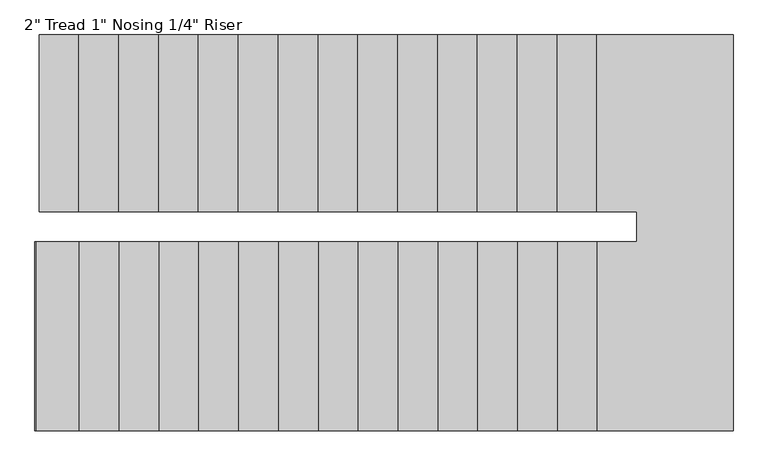
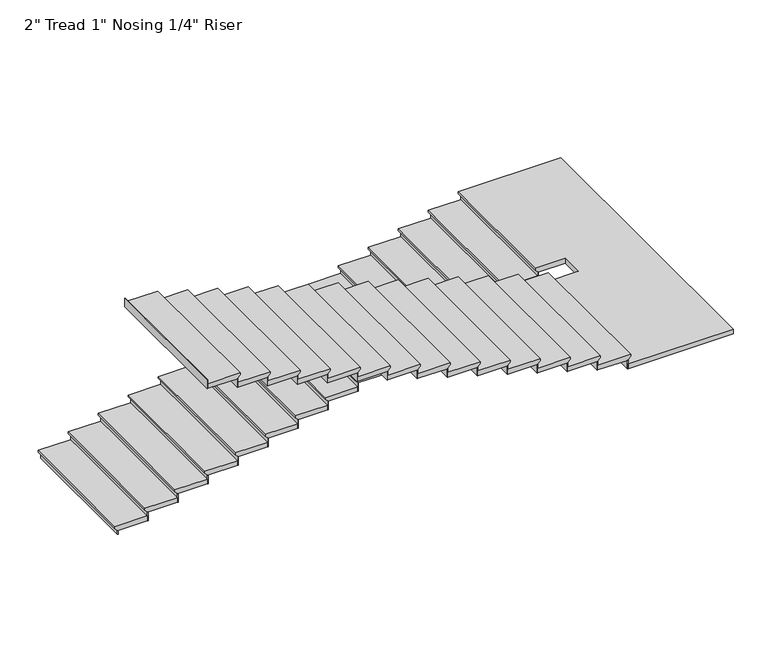
"""IFC4 building model written with IfcOpenShell, lengths in millimetres: stair flight geometry."""

from ifc_helpers import new_model, si_unit, origin, place, context, project, spatial, faceted_brep, source, transform, mapped, element, save


def stair_flight_f74c360e(model_context):
    return source(origin(), model_context, "Body", "Brep", [
        faceted_brep([(-5254.0891351, 11154.2082924, 21408.39), (-5254.0891351, 11154.2082924, 21427.44), (-5254.0891351, 12506.0715905, 21427.44), (-5254.0891351, 12506.0715905, 21408.39), (-5228.6891351, 11154.2082924, 21382.99), (-5228.6891351, 12506.0715905, 21382.99), (-4923.8891351, 11154.2082924, 21427.44), (-4923.8891351, 12506.0715905, 21427.44), (-5228.6891351, 12506.0715905, 21376.64), (-4923.8891351, 12506.0715905, 21376.64), (-4923.8891351, 11154.2082924, 21376.64), (-5228.6891351, 11154.2082924, 21376.64)], [[[0, 1, 2, 3]], [[4, 0, 3, 5]], [[2, 1, 6, 7]], [[8, 9, 10, 11]], [[2, 7, 9, 8, 5, 3]], [[8, 11, 4, 5]], [[6, 1, 0, 4, 11, 10]], [[7, 6, 10, 9]]]),
        faceted_brep([(-5228.6891351, 11154.2082924, 21376.64), (-5228.6891351, 11154.2082924, 21336.0), (-5222.3391351, 11154.2082924, 21336.0), (-5222.3391351, 11154.2082924, 21376.64), (-5228.6891351, 12506.0715905, 21376.64), (-5222.3391351, 12506.0715905, 21376.64), (-5222.3391351, 12506.0715905, 21336.0), (-5228.6891351, 12506.0715905, 21336.0)], [[[0, 1, 2, 3]], [[4, 5, 6, 7]], [[1, 0, 4, 7]], [[2, 1, 7, 6]], [[3, 2, 6, 5]], [[0, 3, 5, 4]]]),
        faceted_brep([(-4923.8891351, 11154.2082924, 21468.08), (-4923.8891351, 11154.2082924, 21376.64), (-4917.5391351, 11154.2082924, 21376.64), (-4917.5391351, 11154.2082924, 21468.08), (-4923.8891351, 12506.0715905, 21468.08), (-4917.5391351, 12506.0715905, 21468.08), (-4917.5391351, 12506.0715905, 21376.64), (-4923.8891351, 12506.0715905, 21376.64)], [[[0, 1, 2, 3]], [[4, 5, 6, 7]], [[1, 0, 4, 7]], [[2, 1, 7, 6]], [[3, 2, 6, 5]], [[0, 3, 5, 4]]]),
        faceted_brep([(-4949.2891351, 12506.0715905, 21518.88), (-4949.2891351, 11154.2082924, 21518.88), (-4619.0891351, 11154.2082924, 21518.88), (-4619.0891351, 12506.0715905, 21518.88), (-4923.8891351, 12506.0715905, 21468.08), (-4619.0891351, 12506.0715905, 21468.08), (-4619.0891351, 11154.2082924, 21468.08), (-4923.8891351, 11154.2082924, 21468.08), (-4923.8891351, 12506.0715905, 21474.43), (-4949.2891351, 12506.0715905, 21499.83), (-4923.8891351, 11154.2082924, 21474.43), (-4949.2891351, 11154.2082924, 21499.83)], [[[0, 1, 2, 3]], [[4, 5, 6, 7]], [[0, 3, 5, 4, 8, 9]], [[4, 7, 10, 8]], [[2, 1, 11, 10, 7, 6]], [[3, 2, 6, 5]], [[11, 1, 0, 9]], [[10, 11, 9, 8]]]),
        faceted_brep([(-4619.0891351, 11154.2082924, 21559.52), (-4619.0891351, 11154.2082924, 21468.08), (-4612.7391351, 11154.2082924, 21468.08), (-4612.7391351, 11154.2082924, 21559.52), (-4619.0891351, 12506.0715905, 21559.52), (-4612.7391351, 12506.0715905, 21559.52), (-4612.7391351, 12506.0715905, 21468.08), (-4619.0891351, 12506.0715905, 21468.08)], [[[0, 1, 2, 3]], [[4, 5, 6, 7]], [[1, 0, 4, 7]], [[2, 1, 7, 6]], [[3, 2, 6, 5]], [[0, 3, 5, 4]]]),
        faceted_brep([(-4644.4891351, 12506.0715905, 21610.32), (-4644.4891351, 11154.2082924, 21610.32), (-4314.2891351, 11154.2082924, 21610.32), (-4314.2891351, 12506.0715905, 21610.32), (-4619.0891351, 12506.0715905, 21559.52), (-4314.2891351, 12506.0715905, 21559.52), (-4314.2891351, 11154.2082924, 21559.52), (-4619.0891351, 11154.2082924, 21559.52), (-4619.0891351, 12506.0715905, 21565.87), (-4644.4891351, 12506.0715905, 21591.27), (-4619.0891351, 11154.2082924, 21565.87), (-4644.4891351, 11154.2082924, 21591.27)], [[[0, 1, 2, 3]], [[4, 5, 6, 7]], [[0, 3, 5, 4, 8, 9]], [[4, 7, 10, 8]], [[2, 1, 11, 10, 7, 6]], [[3, 2, 6, 5]], [[11, 1, 0, 9]], [[10, 11, 9, 8]]]),
        faceted_brep([(-4314.2891351, 11154.2082924, 21650.96), (-4314.2891351, 11154.2082924, 21559.52), (-4307.9391351, 11154.2082924, 21559.52), (-4307.9391351, 11154.2082924, 21650.96), (-4314.2891351, 12506.0715905, 21650.96), (-4307.9391351, 12506.0715905, 21650.96), (-4307.9391351, 12506.0715905, 21559.52), (-4314.2891351, 12506.0715905, 21559.52)], [[[0, 1, 2, 3]], [[4, 5, 6, 7]], [[1, 0, 4, 7]], [[2, 1, 7, 6]], [[3, 2, 6, 5]], [[0, 3, 5, 4]]]),
        faceted_brep([(-4339.6891351, 12506.0715905, 21701.76), (-4339.6891351, 11154.2082924, 21701.76), (-4009.4891351, 11154.2082924, 21701.76), (-4009.4891351, 12506.0715905, 21701.76), (-4314.2891351, 12506.0715905, 21650.96), (-4009.4891351, 12506.0715905, 21650.96), (-4009.4891351, 11154.2082924, 21650.96), (-4314.2891351, 11154.2082924, 21650.96), (-4314.2891351, 12506.0715905, 21657.31), (-4339.6891351, 12506.0715905, 21682.71), (-4314.2891351, 11154.2082924, 21657.31), (-4339.6891351, 11154.2082924, 21682.71)], [[[0, 1, 2, 3]], [[4, 5, 6, 7]], [[0, 3, 5, 4, 8, 9]], [[4, 7, 10, 8]], [[2, 1, 11, 10, 7, 6]], [[3, 2, 6, 5]], [[11, 1, 0, 9]], [[10, 11, 9, 8]]]),
        faceted_brep([(-4009.4891351, 11154.2082924, 21742.4), (-4009.4891351, 11154.2082924, 21650.96), (-4003.1391351, 11154.2082924, 21650.96), (-4003.1391351, 11154.2082924, 21742.4), (-4009.4891351, 12506.0715905, 21742.4), (-4003.1391351, 12506.0715905, 21742.4), (-4003.1391351, 12506.0715905, 21650.96), (-4009.4891351, 12506.0715905, 21650.96)], [[[0, 1, 2, 3]], [[4, 5, 6, 7]], [[1, 0, 4, 7]], [[2, 1, 7, 6]], [[3, 2, 6, 5]], [[0, 3, 5, 4]]]),
        faceted_brep([(-4034.8891351, 12506.0715905, 21793.2), (-4034.8891351, 11154.2082924, 21793.2), (-3704.6891351, 11154.2082924, 21793.2), (-3704.6891351, 12506.0715905, 21793.2), (-4009.4891351, 12506.0715905, 21742.4), (-3704.6891351, 12506.0715905, 21742.4), (-3704.6891351, 11154.2082924, 21742.4), (-4009.4891351, 11154.2082924, 21742.4), (-4009.4891351, 12506.0715905, 21748.75), (-4034.8891351, 12506.0715905, 21774.15), (-4009.4891351, 11154.2082924, 21748.75), (-4034.8891351, 11154.2082924, 21774.15)], [[[0, 1, 2, 3]], [[4, 5, 6, 7]], [[0, 3, 5, 4, 8, 9]], [[4, 7, 10, 8]], [[2, 1, 11, 10, 7, 6]], [[3, 2, 6, 5]], [[11, 1, 0, 9]], [[10, 11, 9, 8]]]),
        faceted_brep([(-3704.6891351, 11154.2082924, 21833.84), (-3704.6891351, 11154.2082924, 21742.4), (-3698.3391351, 11154.2082924, 21742.4), (-3698.3391351, 11154.2082924, 21833.84), (-3704.6891351, 12506.0715905, 21833.84), (-3698.3391351, 12506.0715905, 21833.84), (-3698.3391351, 12506.0715905, 21742.4), (-3704.6891351, 12506.0715905, 21742.4)], [[[0, 1, 2, 3]], [[4, 5, 6, 7]], [[1, 0, 4, 7]], [[2, 1, 7, 6]], [[3, 2, 6, 5]], [[0, 3, 5, 4]]]),
        faceted_brep([(-3730.0891351, 12506.0715905, 21884.64), (-3730.0891351, 11154.2082924, 21884.64), (-3399.8891351, 11154.2082924, 21884.64), (-3399.8891351, 12506.0715905, 21884.64), (-3704.6891351, 12506.0715905, 21833.84), (-3399.8891351, 12506.0715905, 21833.84), (-3399.8891351, 11154.2082924, 21833.84), (-3704.6891351, 11154.2082924, 21833.84), (-3704.6891351, 12506.0715905, 21840.19), (-3730.0891351, 12506.0715905, 21865.59), (-3704.6891351, 11154.2082924, 21840.19), (-3730.0891351, 11154.2082924, 21865.59)], [[[0, 1, 2, 3]], [[4, 5, 6, 7]], [[0, 3, 5, 4, 8, 9]], [[4, 7, 10, 8]], [[2, 1, 11, 10, 7, 6]], [[3, 2, 6, 5]], [[11, 1, 0, 9]], [[10, 11, 9, 8]]]),
        faceted_brep([(-3399.8891351, 11154.2082924, 21925.28), (-3399.8891351, 11154.2082924, 21833.84), (-3393.5391351, 11154.2082924, 21833.84), (-3393.5391351, 11154.2082924, 21925.28), (-3399.8891351, 12506.0715905, 21925.28), (-3393.5391351, 12506.0715905, 21925.28), (-3393.5391351, 12506.0715905, 21833.84), (-3399.8891351, 12506.0715905, 21833.84)], [[[0, 1, 2, 3]], [[4, 5, 6, 7]], [[1, 0, 4, 7]], [[2, 1, 7, 6]], [[3, 2, 6, 5]], [[0, 3, 5, 4]]]),
        faceted_brep([(-3425.2891351, 12506.0715905, 21976.08), (-3425.2891351, 11154.2082924, 21976.08), (-3095.0891351, 11154.2082924, 21976.08), (-3095.0891351, 12506.0715905, 21976.08), (-3399.8891351, 12506.0715905, 21925.28), (-3095.0891351, 12506.0715905, 21925.28), (-3095.0891351, 11154.2082924, 21925.28), (-3399.8891351, 11154.2082924, 21925.28), (-3399.8891351, 12506.0715905, 21931.63), (-3425.2891351, 12506.0715905, 21957.03), (-3399.8891351, 11154.2082924, 21931.63), (-3425.2891351, 11154.2082924, 21957.03)], [[[0, 1, 2, 3]], [[4, 5, 6, 7]], [[0, 3, 5, 4, 8, 9]], [[4, 7, 10, 8]], [[2, 1, 11, 10, 7, 6]], [[3, 2, 6, 5]], [[11, 1, 0, 9]], [[10, 11, 9, 8]]]),
        faceted_brep([(-3095.0891351, 11154.2082924, 22016.72), (-3095.0891351, 11154.2082924, 21925.28), (-3088.7391351, 11154.2082924, 21925.28), (-3088.7391351, 11154.2082924, 22016.72), (-3095.0891351, 12506.0715905, 22016.72), (-3088.7391351, 12506.0715905, 22016.72), (-3088.7391351, 12506.0715905, 21925.28), (-3095.0891351, 12506.0715905, 21925.28)], [[[0, 1, 2, 3]], [[4, 5, 6, 7]], [[1, 0, 4, 7]], [[2, 1, 7, 6]], [[3, 2, 6, 5]], [[0, 3, 5, 4]]]),
        faceted_brep([(-3120.4891351, 12506.0715905, 22067.52), (-3120.4891351, 11154.2082924, 22067.52), (-2790.2891351, 11154.2082924, 22067.52), (-2790.2891351, 12506.0715905, 22067.52), (-3095.0891351, 12506.0715905, 22016.72), (-2790.2891351, 12506.0715905, 22016.72), (-2790.2891351, 11154.2082924, 22016.72), (-3095.0891351, 11154.2082924, 22016.72), (-3095.0891351, 12506.0715905, 22023.07), (-3120.4891351, 12506.0715905, 22048.47), (-3095.0891351, 11154.2082924, 22023.07), (-3120.4891351, 11154.2082924, 22048.47)], [[[0, 1, 2, 3]], [[4, 5, 6, 7]], [[0, 3, 5, 4, 8, 9]], [[4, 7, 10, 8]], [[2, 1, 11, 10, 7, 6]], [[3, 2, 6, 5]], [[11, 1, 0, 9]], [[10, 11, 9, 8]]]),
        faceted_brep([(-2790.2891351, 11154.2082924, 22108.16), (-2790.2891351, 11154.2082924, 22016.72), (-2783.9391351, 11154.2082924, 22016.72), (-2783.9391351, 11154.2082924, 22108.16), (-2790.2891351, 12506.0715905, 22108.16), (-2783.9391351, 12506.0715905, 22108.16), (-2783.9391351, 12506.0715905, 22016.72), (-2790.2891351, 12506.0715905, 22016.72)], [[[0, 1, 2, 3]], [[4, 5, 6, 7]], [[1, 0, 4, 7]], [[2, 1, 7, 6]], [[3, 2, 6, 5]], [[0, 3, 5, 4]]]),
        faceted_brep([(-2815.6891351, 12506.0715905, 22158.96), (-2815.6891351, 11154.2082924, 22158.96), (-2485.4891351, 11154.2082924, 22158.96), (-2485.4891351, 12506.0715905, 22158.96), (-2790.2891351, 12506.0715905, 22108.16), (-2485.4891351, 12506.0715905, 22108.16), (-2485.4891351, 11154.2082924, 22108.16), (-2790.2891351, 11154.2082924, 22108.16), (-2790.2891351, 12506.0715905, 22114.51), (-2815.6891351, 12506.0715905, 22139.91), (-2790.2891351, 11154.2082924, 22114.51), (-2815.6891351, 11154.2082924, 22139.91)], [[[0, 1, 2, 3]], [[4, 5, 6, 7]], [[0, 3, 5, 4, 8, 9]], [[4, 7, 10, 8]], [[2, 1, 11, 10, 7, 6]], [[3, 2, 6, 5]], [[11, 1, 0, 9]], [[10, 11, 9, 8]]]),
        faceted_brep([(-2485.4891351, 11154.2082924, 22199.6), (-2485.4891351, 11154.2082924, 22108.16), (-2479.1391351, 11154.2082924, 22108.16), (-2479.1391351, 11154.2082924, 22199.6), (-2485.4891351, 12506.0715905, 22199.6), (-2479.1391351, 12506.0715905, 22199.6), (-2479.1391351, 12506.0715905, 22108.16), (-2485.4891351, 12506.0715905, 22108.16)], [[[0, 1, 2, 3]], [[4, 5, 6, 7]], [[1, 0, 4, 7]], [[2, 1, 7, 6]], [[3, 2, 6, 5]], [[0, 3, 5, 4]]]),
        faceted_brep([(-2510.8891351, 12506.0715905, 22250.4), (-2510.8891351, 11154.2082924, 22250.4), (-2180.6891351, 11154.2082924, 22250.4), (-2180.6891351, 12506.0715905, 22250.4), (-2485.4891351, 12506.0715905, 22199.6), (-2180.6891351, 12506.0715905, 22199.6), (-2180.6891351, 11154.2082924, 22199.6), (-2485.4891351, 11154.2082924, 22199.6), (-2485.4891351, 12506.0715905, 22205.95), (-2510.8891351, 12506.0715905, 22231.35), (-2485.4891351, 11154.2082924, 22205.95), (-2510.8891351, 11154.2082924, 22231.35)], [[[0, 1, 2, 3]], [[4, 5, 6, 7]], [[0, 3, 5, 4, 8, 9]], [[4, 7, 10, 8]], [[2, 1, 11, 10, 7, 6]], [[3, 2, 6, 5]], [[11, 1, 0, 9]], [[10, 11, 9, 8]]]),
        faceted_brep([(-2180.6891351, 11154.2082924, 22291.04), (-2180.6891351, 11154.2082924, 22199.6), (-2174.3391351, 11154.2082924, 22199.6), (-2174.3391351, 11154.2082924, 22291.04), (-2180.6891351, 12506.0715905, 22291.04), (-2174.3391351, 12506.0715905, 22291.04), (-2174.3391351, 12506.0715905, 22199.6), (-2180.6891351, 12506.0715905, 22199.6)], [[[0, 1, 2, 3]], [[4, 5, 6, 7]], [[1, 0, 4, 7]], [[2, 1, 7, 6]], [[3, 2, 6, 5]], [[0, 3, 5, 4]]]),
        faceted_brep([(-2206.0891351, 12506.0715905, 22341.84), (-2206.0891351, 11154.2082924, 22341.84), (-1875.8891351, 11154.2082924, 22341.84), (-1875.8891351, 12506.0715905, 22341.84), (-2180.6891351, 12506.0715905, 22291.04), (-1875.8891351, 12506.0715905, 22291.04), (-1875.8891351, 11154.2082924, 22291.04), (-2180.6891351, 11154.2082924, 22291.04), (-2180.6891351, 12506.0715905, 22297.39), (-2206.0891351, 12506.0715905, 22322.79), (-2180.6891351, 11154.2082924, 22297.39), (-2206.0891351, 11154.2082924, 22322.79)], [[[0, 1, 2, 3]], [[4, 5, 6, 7]], [[0, 3, 5, 4, 8, 9]], [[4, 7, 10, 8]], [[2, 1, 11, 10, 7, 6]], [[3, 2, 6, 5]], [[11, 1, 0, 9]], [[10, 11, 9, 8]]]),
        faceted_brep([(-1875.8891351, 11154.2082924, 22382.48), (-1875.8891351, 11154.2082924, 22291.04), (-1869.5391351, 11154.2082924, 22291.04), (-1869.5391351, 11154.2082924, 22382.48), (-1875.8891351, 12506.0715905, 22382.48), (-1869.5391351, 12506.0715905, 22382.48), (-1869.5391351, 12506.0715905, 22291.04), (-1875.8891351, 12506.0715905, 22291.04)], [[[0, 1, 2, 3]], [[4, 5, 6, 7]], [[1, 0, 4, 7]], [[2, 1, 7, 6]], [[3, 2, 6, 5]], [[0, 3, 5, 4]]]),
        faceted_brep([(-1901.2891351, 12506.0715905, 22433.28), (-1901.2891351, 11154.2082924, 22433.28), (-1571.0891351, 11154.2082924, 22433.28), (-1571.0891351, 12506.0715905, 22433.28), (-1875.8891351, 12506.0715905, 22382.48), (-1571.0891351, 12506.0715905, 22382.48), (-1571.0891351, 11154.2082924, 22382.48), (-1875.8891351, 11154.2082924, 22382.48), (-1875.8891351, 12506.0715905, 22388.83), (-1901.2891351, 12506.0715905, 22414.23), (-1875.8891351, 11154.2082924, 22388.83), (-1901.2891351, 11154.2082924, 22414.23)], [[[0, 1, 2, 3]], [[4, 5, 6, 7]], [[0, 3, 5, 4, 8, 9]], [[4, 7, 10, 8]], [[2, 1, 11, 10, 7, 6]], [[3, 2, 6, 5]], [[11, 1, 0, 9]], [[10, 11, 9, 8]]]),
        faceted_brep([(-1571.0891351, 11154.2082924, 22473.92), (-1571.0891351, 11154.2082924, 22382.48), (-1564.7391351, 11154.2082924, 22382.48), (-1564.7391351, 11154.2082924, 22473.92), (-1571.0891351, 12506.0715905, 22473.92), (-1564.7391351, 12506.0715905, 22473.92), (-1564.7391351, 12506.0715905, 22382.48), (-1571.0891351, 12506.0715905, 22382.48)], [[[0, 1, 2, 3]], [[4, 5, 6, 7]], [[1, 0, 4, 7]], [[2, 1, 7, 6]], [[3, 2, 6, 5]], [[0, 3, 5, 4]]]),
        faceted_brep([(-1596.4891351, 12506.0715905, 22524.72), (-1596.4891351, 11154.2082924, 22524.72), (-1266.2891351, 11154.2082924, 22524.72), (-1266.2891351, 12506.0715905, 22524.72), (-1571.0891351, 12506.0715905, 22473.92), (-1266.2891351, 12506.0715905, 22473.92), (-1266.2891351, 11154.2082924, 22473.92), (-1571.0891351, 11154.2082924, 22473.92), (-1571.0891351, 12506.0715905, 22480.27), (-1596.4891351, 12506.0715905, 22505.67), (-1571.0891351, 11154.2082924, 22480.27), (-1596.4891351, 11154.2082924, 22505.67)], [[[0, 1, 2, 3]], [[4, 5, 6, 7]], [[0, 3, 5, 4, 8, 9]], [[4, 7, 10, 8]], [[2, 1, 11, 10, 7, 6]], [[3, 2, 6, 5]], [[11, 1, 0, 9]], [[10, 11, 9, 8]]]),
        faceted_brep([(-1266.2891351, 11154.2082924, 22565.36), (-1266.2891351, 11154.2082924, 22473.92), (-1259.9391351, 11154.2082924, 22473.92), (-1259.9391351, 11154.2082924, 22565.36), (-1266.2891351, 12506.0715905, 22565.36), (-1259.9391351, 12506.0715905, 22565.36), (-1259.9391351, 12506.0715905, 22473.92), (-1266.2891351, 12506.0715905, 22473.92)], [[[0, 1, 2, 3]], [[4, 5, 6, 7]], [[1, 0, 4, 7]], [[2, 1, 7, 6]], [[3, 2, 6, 5]], [[0, 3, 5, 4]]]),
        faceted_brep([(-1291.6891351, 12506.0715905, 22616.16), (-1291.6891351, 11154.2082924, 22616.16), (-961.4891351, 11154.2082924, 22616.16), (-961.4891351, 12506.0715905, 22616.16), (-1266.2891351, 12506.0715905, 22565.36), (-961.4891351, 12506.0715905, 22565.36), (-961.4891351, 11154.2082924, 22565.36), (-1266.2891351, 11154.2082924, 22565.36), (-1266.2891351, 12506.0715905, 22571.71), (-1291.6891351, 12506.0715905, 22597.11), (-1266.2891351, 11154.2082924, 22571.71), (-1291.6891351, 11154.2082924, 22597.11)], [[[0, 1, 2, 3]], [[4, 5, 6, 7]], [[0, 3, 5, 4, 8, 9]], [[4, 7, 10, 8]], [[2, 1, 11, 10, 7, 6]], [[3, 2, 6, 5]], [[11, 1, 0, 9]], [[10, 11, 9, 8]]]),
        faceted_brep([(-961.4891351, 11154.2082924, 22656.8), (-961.4891351, 11154.2082924, 22565.36), (-955.1391351, 11154.2082924, 22565.36), (-955.1391351, 11154.2082924, 22656.8), (-961.4891351, 12506.0715905, 22656.8), (-955.1391351, 12506.0715905, 22656.8), (-955.1391351, 12506.0715905, 22565.36), (-961.4891351, 12506.0715905, 22565.36)], [[[0, 1, 2, 3]], [[4, 5, 6, 7]], [[1, 0, 4, 7]], [[2, 1, 7, 6]], [[3, 2, 6, 5]], [[0, 3, 5, 4]]]),
        faceted_brep([(-1012.2891351, 9478.4949943, 22707.6), (54.5108649, 9478.4949943, 22707.6), (54.5108649, 12506.0715905, 22707.6), (-986.8891351, 12506.0715905, 22707.6), (-986.8891351, 11154.2082924, 22707.6), (-682.0891351, 11154.2082924, 22707.6), (-682.0891351, 10925.6082924, 22707.6), (-1012.2891351, 10925.6082924, 22707.6), (54.5108649, 9478.4949943, 22656.8), (-1012.2891351, 9478.4949943, 22656.8), (-1012.2891351, 10925.6082924, 22656.8), (-682.0891351, 10925.6082924, 22656.8), (-682.0891351, 11154.2082924, 22656.8), (-961.4891351, 11154.2082924, 22656.8), (-961.4891351, 12506.0715905, 22656.8), (54.5108649, 12506.0715905, 22656.8), (-961.4891351, 12506.0715905, 22663.15), (-986.8891351, 12506.0715905, 22688.55), (-961.4891351, 11154.2082924, 22663.15), (-986.8891351, 11154.2082924, 22688.55)], [[[0, 1, 2, 3, 4, 5, 6, 7]], [[8, 9, 10, 11, 12, 13, 14, 15]], [[1, 0, 9, 8]], [[2, 1, 8, 15]], [[3, 2, 15, 14, 16, 17]], [[14, 13, 18, 16]], [[5, 4, 19, 18, 13, 12]], [[6, 5, 12, 11]], [[7, 6, 11, 10]], [[0, 7, 10, 9]], [[19, 4, 3, 17]], [[18, 19, 17, 16]]]),
        faceted_brep([(-1012.2891351, 10925.6082924, 22748.24), (-1012.2891351, 10925.6082924, 22656.8), (-1018.6391351, 10925.6082924, 22656.8), (-1018.6391351, 10925.6082924, 22748.24), (-1012.2891351, 9478.4949943, 22748.24), (-1018.6391351, 9478.4949943, 22748.24), (-1018.6391351, 9478.4949943, 22656.8), (-1012.2891351, 9478.4949943, 22656.8)], [[[0, 1, 2, 3]], [[4, 5, 6, 7]], [[1, 0, 4, 7]], [[2, 1, 7, 6]], [[3, 2, 6, 5]], [[0, 3, 5, 4]]]),
        faceted_brep([(-986.8891351, 9478.4949943, 22799.04), (-986.8891351, 10925.6082924, 22799.04), (-1317.0891351, 10925.6082924, 22799.04), (-1317.0891351, 9478.4949943, 22799.04), (-1012.2891351, 9478.4949943, 22748.24), (-1317.0891351, 9478.4949943, 22748.24), (-1317.0891351, 10925.6082924, 22748.24), (-1012.2891351, 10925.6082924, 22748.24), (-1012.2891351, 9478.4949943, 22754.59), (-986.8891351, 9478.4949943, 22779.99), (-1012.2891351, 10925.6082924, 22754.59), (-986.8891351, 10925.6082924, 22779.99)], [[[0, 1, 2, 3]], [[4, 5, 6, 7]], [[0, 3, 5, 4, 8, 9]], [[4, 7, 10, 8]], [[2, 1, 11, 10, 7, 6]], [[3, 2, 6, 5]], [[11, 1, 0, 9]], [[10, 11, 9, 8]]]),
        faceted_brep([(-1317.0891351, 10925.6082924, 22839.68), (-1317.0891351, 10925.6082924, 22748.24), (-1323.4391351, 10925.6082924, 22748.24), (-1323.4391351, 10925.6082924, 22839.68), (-1317.0891351, 9478.4949943, 22839.68), (-1323.4391351, 9478.4949943, 22839.68), (-1323.4391351, 9478.4949943, 22748.24), (-1317.0891351, 9478.4949943, 22748.24)], [[[0, 1, 2, 3]], [[4, 5, 6, 7]], [[1, 0, 4, 7]], [[2, 1, 7, 6]], [[3, 2, 6, 5]], [[0, 3, 5, 4]]]),
        faceted_brep([(-1291.6891351, 9478.4949943, 22890.48), (-1291.6891351, 10925.6082924, 22890.48), (-1621.8891351, 10925.6082924, 22890.48), (-1621.8891351, 9478.4949943, 22890.48), (-1317.0891351, 9478.4949943, 22839.68), (-1621.8891351, 9478.4949943, 22839.68), (-1621.8891351, 10925.6082924, 22839.68), (-1317.0891351, 10925.6082924, 22839.68), (-1317.0891351, 9478.4949943, 22846.03), (-1291.6891351, 9478.4949943, 22871.43), (-1317.0891351, 10925.6082924, 22846.03), (-1291.6891351, 10925.6082924, 22871.43)], [[[0, 1, 2, 3]], [[4, 5, 6, 7]], [[0, 3, 5, 4, 8, 9]], [[4, 7, 10, 8]], [[2, 1, 11, 10, 7, 6]], [[3, 2, 6, 5]], [[11, 1, 0, 9]], [[10, 11, 9, 8]]]),
        faceted_brep([(-1621.8891351, 10925.6082924, 22931.12), (-1621.8891351, 10925.6082924, 22839.68), (-1628.2391351, 10925.6082924, 22839.68), (-1628.2391351, 10925.6082924, 22931.12), (-1621.8891351, 9478.4949943, 22931.12), (-1628.2391351, 9478.4949943, 22931.12), (-1628.2391351, 9478.4949943, 22839.68), (-1621.8891351, 9478.4949943, 22839.68)], [[[0, 1, 2, 3]], [[4, 5, 6, 7]], [[1, 0, 4, 7]], [[2, 1, 7, 6]], [[3, 2, 6, 5]], [[0, 3, 5, 4]]]),
        faceted_brep([(-1596.4891351, 9478.4949943, 22981.92), (-1596.4891351, 10925.6082924, 22981.92), (-1926.6891351, 10925.6082924, 22981.92), (-1926.6891351, 9478.4949943, 22981.92), (-1621.8891351, 9478.4949943, 22931.12), (-1926.6891351, 9478.4949943, 22931.12), (-1926.6891351, 10925.6082924, 22931.12), (-1621.8891351, 10925.6082924, 22931.12), (-1621.8891351, 9478.4949943, 22937.47), (-1596.4891351, 9478.4949943, 22962.87), (-1621.8891351, 10925.6082924, 22937.47), (-1596.4891351, 10925.6082924, 22962.87)], [[[0, 1, 2, 3]], [[4, 5, 6, 7]], [[0, 3, 5, 4, 8, 9]], [[4, 7, 10, 8]], [[2, 1, 11, 10, 7, 6]], [[3, 2, 6, 5]], [[11, 1, 0, 9]], [[10, 11, 9, 8]]]),
        faceted_brep([(-1926.6891351, 10925.6082924, 23022.56), (-1926.6891351, 10925.6082924, 22931.12), (-1933.0391351, 10925.6082924, 22931.12), (-1933.0391351, 10925.6082924, 23022.56), (-1926.6891351, 9478.4949943, 23022.56), (-1933.0391351, 9478.4949943, 23022.56), (-1933.0391351, 9478.4949943, 22931.12), (-1926.6891351, 9478.4949943, 22931.12)], [[[0, 1, 2, 3]], [[4, 5, 6, 7]], [[1, 0, 4, 7]], [[2, 1, 7, 6]], [[3, 2, 6, 5]], [[0, 3, 5, 4]]]),
        faceted_brep([(-1901.2891351, 9478.4949943, 23073.36), (-1901.2891351, 10925.6082924, 23073.36), (-2231.4891351, 10925.6082924, 23073.36), (-2231.4891351, 9478.4949943, 23073.36), (-1926.6891351, 9478.4949943, 23022.56), (-2231.4891351, 9478.4949943, 23022.56), (-2231.4891351, 10925.6082924, 23022.56), (-1926.6891351, 10925.6082924, 23022.56), (-1926.6891351, 9478.4949943, 23028.91), (-1901.2891351, 9478.4949943, 23054.31), (-1926.6891351, 10925.6082924, 23028.91), (-1901.2891351, 10925.6082924, 23054.31)], [[[0, 1, 2, 3]], [[4, 5, 6, 7]], [[0, 3, 5, 4, 8, 9]], [[4, 7, 10, 8]], [[2, 1, 11, 10, 7, 6]], [[3, 2, 6, 5]], [[11, 1, 0, 9]], [[10, 11, 9, 8]]]),
        faceted_brep([(-2231.4891351, 10925.6082924, 23114.0), (-2231.4891351, 10925.6082924, 23022.56), (-2237.8391351, 10925.6082924, 23022.56), (-2237.8391351, 10925.6082924, 23114.0), (-2231.4891351, 9478.4949943, 23114.0), (-2237.8391351, 9478.4949943, 23114.0), (-2237.8391351, 9478.4949943, 23022.56), (-2231.4891351, 9478.4949943, 23022.56)], [[[0, 1, 2, 3]], [[4, 5, 6, 7]], [[1, 0, 4, 7]], [[2, 1, 7, 6]], [[3, 2, 6, 5]], [[0, 3, 5, 4]]]),
        faceted_brep([(-2206.0891351, 9478.4949943, 23164.8), (-2206.0891351, 10925.6082924, 23164.8), (-2536.2891351, 10925.6082924, 23164.8), (-2536.2891351, 9478.4949943, 23164.8), (-2231.4891351, 9478.4949943, 23114.0), (-2536.2891351, 9478.4949943, 23114.0), (-2536.2891351, 10925.6082924, 23114.0), (-2231.4891351, 10925.6082924, 23114.0), (-2231.4891351, 9478.4949943, 23120.35), (-2206.0891351, 9478.4949943, 23145.75), (-2231.4891351, 10925.6082924, 23120.35), (-2206.0891351, 10925.6082924, 23145.75)], [[[0, 1, 2, 3]], [[4, 5, 6, 7]], [[0, 3, 5, 4, 8, 9]], [[4, 7, 10, 8]], [[2, 1, 11, 10, 7, 6]], [[3, 2, 6, 5]], [[11, 1, 0, 9]], [[10, 11, 9, 8]]]),
        faceted_brep([(-2536.2891351, 10925.6082924, 23205.44), (-2536.2891351, 10925.6082924, 23114.0), (-2542.6391351, 10925.6082924, 23114.0), (-2542.6391351, 10925.6082924, 23205.44), (-2536.2891351, 9478.4949943, 23205.44), (-2542.6391351, 9478.4949943, 23205.44), (-2542.6391351, 9478.4949943, 23114.0), (-2536.2891351, 9478.4949943, 23114.0)], [[[0, 1, 2, 3]], [[4, 5, 6, 7]], [[1, 0, 4, 7]], [[2, 1, 7, 6]], [[3, 2, 6, 5]], [[0, 3, 5, 4]]]),
        faceted_brep([(-2510.8891351, 9478.4949943, 23256.24), (-2510.8891351, 10925.6082924, 23256.24), (-2841.0891351, 10925.6082924, 23256.24), (-2841.0891351, 9478.4949943, 23256.24), (-2536.2891351, 9478.4949943, 23205.44), (-2841.0891351, 9478.4949943, 23205.44), (-2841.0891351, 10925.6082924, 23205.44), (-2536.2891351, 10925.6082924, 23205.44), (-2536.2891351, 9478.4949943, 23211.79), (-2510.8891351, 9478.4949943, 23237.19), (-2536.2891351, 10925.6082924, 23211.79), (-2510.8891351, 10925.6082924, 23237.19)], [[[0, 1, 2, 3]], [[4, 5, 6, 7]], [[0, 3, 5, 4, 8, 9]], [[4, 7, 10, 8]], [[2, 1, 11, 10, 7, 6]], [[3, 2, 6, 5]], [[11, 1, 0, 9]], [[10, 11, 9, 8]]]),
        faceted_brep([(-2841.0891351, 10925.6082924, 23296.88), (-2841.0891351, 10925.6082924, 23205.44), (-2847.4391351, 10925.6082924, 23205.44), (-2847.4391351, 10925.6082924, 23296.88), (-2841.0891351, 9478.4949943, 23296.88), (-2847.4391351, 9478.4949943, 23296.88), (-2847.4391351, 9478.4949943, 23205.44), (-2841.0891351, 9478.4949943, 23205.44)], [[[0, 1, 2, 3]], [[4, 5, 6, 7]], [[1, 0, 4, 7]], [[2, 1, 7, 6]], [[3, 2, 6, 5]], [[0, 3, 5, 4]]]),
        faceted_brep([(-2815.6891351, 9478.4949943, 23347.68), (-2815.6891351, 10925.6082924, 23347.68), (-3145.8891351, 10925.6082924, 23347.68), (-3145.8891351, 9478.4949943, 23347.68), (-2841.0891351, 9478.4949943, 23296.88), (-3145.8891351, 9478.4949943, 23296.88), (-3145.8891351, 10925.6082924, 23296.88), (-2841.0891351, 10925.6082924, 23296.88), (-2841.0891351, 9478.4949943, 23303.23), (-2815.6891351, 9478.4949943, 23328.63), (-2841.0891351, 10925.6082924, 23303.23), (-2815.6891351, 10925.6082924, 23328.63)], [[[0, 1, 2, 3]], [[4, 5, 6, 7]], [[0, 3, 5, 4, 8, 9]], [[4, 7, 10, 8]], [[2, 1, 11, 10, 7, 6]], [[3, 2, 6, 5]], [[11, 1, 0, 9]], [[10, 11, 9, 8]]]),
        faceted_brep([(-3145.8891351, 10925.6082924, 23388.32), (-3145.8891351, 10925.6082924, 23296.88), (-3152.2391351, 10925.6082924, 23296.88), (-3152.2391351, 10925.6082924, 23388.32), (-3145.8891351, 9478.4949943, 23388.32), (-3152.2391351, 9478.4949943, 23388.32), (-3152.2391351, 9478.4949943, 23296.88), (-3145.8891351, 9478.4949943, 23296.88)], [[[0, 1, 2, 3]], [[4, 5, 6, 7]], [[1, 0, 4, 7]], [[2, 1, 7, 6]], [[3, 2, 6, 5]], [[0, 3, 5, 4]]]),
        faceted_brep([(-3120.4891351, 9478.4949943, 23439.12), (-3120.4891351, 10925.6082924, 23439.12), (-3450.6891351, 10925.6082924, 23439.12), (-3450.6891351, 9478.4949943, 23439.12), (-3145.8891351, 9478.4949943, 23388.32), (-3450.6891351, 9478.4949943, 23388.32), (-3450.6891351, 10925.6082924, 23388.32), (-3145.8891351, 10925.6082924, 23388.32), (-3145.8891351, 9478.4949943, 23394.67), (-3120.4891351, 9478.4949943, 23420.07), (-3145.8891351, 10925.6082924, 23394.67), (-3120.4891351, 10925.6082924, 23420.07)], [[[0, 1, 2, 3]], [[4, 5, 6, 7]], [[0, 3, 5, 4, 8, 9]], [[4, 7, 10, 8]], [[2, 1, 11, 10, 7, 6]], [[3, 2, 6, 5]], [[11, 1, 0, 9]], [[10, 11, 9, 8]]]),
        faceted_brep([(-3450.6891351, 10925.6082924, 23479.76), (-3450.6891351, 10925.6082924, 23388.32), (-3457.0391351, 10925.6082924, 23388.32), (-3457.0391351, 10925.6082924, 23479.76), (-3450.6891351, 9478.4949943, 23479.76), (-3457.0391351, 9478.4949943, 23479.76), (-3457.0391351, 9478.4949943, 23388.32), (-3450.6891351, 9478.4949943, 23388.32)], [[[0, 1, 2, 3]], [[4, 5, 6, 7]], [[1, 0, 4, 7]], [[2, 1, 7, 6]], [[3, 2, 6, 5]], [[0, 3, 5, 4]]]),
        faceted_brep([(-3425.2891351, 9478.4949943, 23530.56), (-3425.2891351, 10925.6082924, 23530.56), (-3755.4891351, 10925.6082924, 23530.56), (-3755.4891351, 9478.4949943, 23530.56), (-3450.6891351, 9478.4949943, 23479.76), (-3755.4891351, 9478.4949943, 23479.76), (-3755.4891351, 10925.6082924, 23479.76), (-3450.6891351, 10925.6082924, 23479.76), (-3450.6891351, 9478.4949943, 23486.11), (-3425.2891351, 9478.4949943, 23511.51), (-3450.6891351, 10925.6082924, 23486.11), (-3425.2891351, 10925.6082924, 23511.51)], [[[0, 1, 2, 3]], [[4, 5, 6, 7]], [[0, 3, 5, 4, 8, 9]], [[4, 7, 10, 8]], [[2, 1, 11, 10, 7, 6]], [[3, 2, 6, 5]], [[11, 1, 0, 9]], [[10, 11, 9, 8]]]),
        faceted_brep([(-3755.4891351, 10925.6082924, 23571.2), (-3755.4891351, 10925.6082924, 23479.76), (-3761.8391351, 10925.6082924, 23479.76), (-3761.8391351, 10925.6082924, 23571.2), (-3755.4891351, 9478.4949943, 23571.2), (-3761.8391351, 9478.4949943, 23571.2), (-3761.8391351, 9478.4949943, 23479.76), (-3755.4891351, 9478.4949943, 23479.76)], [[[0, 1, 2, 3]], [[4, 5, 6, 7]], [[1, 0, 4, 7]], [[2, 1, 7, 6]], [[3, 2, 6, 5]], [[0, 3, 5, 4]]]),
        faceted_brep([(-3730.0891351, 9478.4949943, 23622.0), (-3730.0891351, 10925.6082924, 23622.0), (-4060.2891351, 10925.6082924, 23622.0), (-4060.2891351, 9478.4949943, 23622.0), (-3755.4891351, 9478.4949943, 23571.2), (-4060.2891351, 9478.4949943, 23571.2), (-4060.2891351, 10925.6082924, 23571.2), (-3755.4891351, 10925.6082924, 23571.2), (-3755.4891351, 9478.4949943, 23577.55), (-3730.0891351, 9478.4949943, 23602.95), (-3755.4891351, 10925.6082924, 23577.55), (-3730.0891351, 10925.6082924, 23602.95)], [[[0, 1, 2, 3]], [[4, 5, 6, 7]], [[0, 3, 5, 4, 8, 9]], [[4, 7, 10, 8]], [[2, 1, 11, 10, 7, 6]], [[3, 2, 6, 5]], [[11, 1, 0, 9]], [[10, 11, 9, 8]]]),
        faceted_brep([(-4060.2891351, 10925.6082924, 23662.64), (-4060.2891351, 10925.6082924, 23571.2), (-4066.6391351, 10925.6082924, 23571.2), (-4066.6391351, 10925.6082924, 23662.64), (-4060.2891351, 9478.4949943, 23662.64), (-4066.6391351, 9478.4949943, 23662.64), (-4066.6391351, 9478.4949943, 23571.2), (-4060.2891351, 9478.4949943, 23571.2)], [[[0, 1, 2, 3]], [[4, 5, 6, 7]], [[1, 0, 4, 7]], [[2, 1, 7, 6]], [[3, 2, 6, 5]], [[0, 3, 5, 4]]]),
        faceted_brep([(-4034.8891351, 9478.4949943, 23713.44), (-4034.8891351, 10925.6082924, 23713.44), (-4365.0891351, 10925.6082924, 23713.44), (-4365.0891351, 9478.4949943, 23713.44), (-4060.2891351, 9478.4949943, 23662.64), (-4365.0891351, 9478.4949943, 23662.64), (-4365.0891351, 10925.6082924, 23662.64), (-4060.2891351, 10925.6082924, 23662.64), (-4060.2891351, 9478.4949943, 23668.99), (-4034.8891351, 9478.4949943, 23694.39), (-4060.2891351, 10925.6082924, 23668.99), (-4034.8891351, 10925.6082924, 23694.39)], [[[0, 1, 2, 3]], [[4, 5, 6, 7]], [[0, 3, 5, 4, 8, 9]], [[4, 7, 10, 8]], [[2, 1, 11, 10, 7, 6]], [[3, 2, 6, 5]], [[11, 1, 0, 9]], [[10, 11, 9, 8]]]),
        faceted_brep([(-4365.0891351, 10925.6082924, 23754.08), (-4365.0891351, 10925.6082924, 23662.64), (-4371.4391351, 10925.6082924, 23662.64), (-4371.4391351, 10925.6082924, 23754.08), (-4365.0891351, 9478.4949943, 23754.08), (-4371.4391351, 9478.4949943, 23754.08), (-4371.4391351, 9478.4949943, 23662.64), (-4365.0891351, 9478.4949943, 23662.64)], [[[0, 1, 2, 3]], [[4, 5, 6, 7]], [[1, 0, 4, 7]], [[2, 1, 7, 6]], [[3, 2, 6, 5]], [[0, 3, 5, 4]]]),
        faceted_brep([(-4339.6891351, 9478.4949943, 23804.88), (-4339.6891351, 10925.6082924, 23804.88), (-4669.8891351, 10925.6082924, 23804.88), (-4669.8891351, 9478.4949943, 23804.88), (-4365.0891351, 9478.4949943, 23754.08), (-4669.8891351, 9478.4949943, 23754.08), (-4669.8891351, 10925.6082924, 23754.08), (-4365.0891351, 10925.6082924, 23754.08), (-4365.0891351, 9478.4949943, 23760.43), (-4339.6891351, 9478.4949943, 23785.83), (-4365.0891351, 10925.6082924, 23760.43), (-4339.6891351, 10925.6082924, 23785.83)], [[[0, 1, 2, 3]], [[4, 5, 6, 7]], [[0, 3, 5, 4, 8, 9]], [[4, 7, 10, 8]], [[2, 1, 11, 10, 7, 6]], [[3, 2, 6, 5]], [[11, 1, 0, 9]], [[10, 11, 9, 8]]]),
        faceted_brep([(-4669.8891351, 10925.6082924, 23845.52), (-4669.8891351, 10925.6082924, 23754.08), (-4676.2391351, 10925.6082924, 23754.08), (-4676.2391351, 10925.6082924, 23845.52), (-4669.8891351, 9478.4949943, 23845.52), (-4676.2391351, 9478.4949943, 23845.52), (-4676.2391351, 9478.4949943, 23754.08), (-4669.8891351, 9478.4949943, 23754.08)], [[[0, 1, 2, 3]], [[4, 5, 6, 7]], [[1, 0, 4, 7]], [[2, 1, 7, 6]], [[3, 2, 6, 5]], [[0, 3, 5, 4]]]),
        faceted_brep([(-4644.4891351, 9478.4949943, 23896.32), (-4644.4891351, 10925.6082924, 23896.32), (-4974.6891351, 10925.6082924, 23896.32), (-4974.6891351, 9478.4949943, 23896.32), (-4669.8891351, 9478.4949943, 23845.52), (-4974.6891351, 9478.4949943, 23845.52), (-4974.6891351, 10925.6082924, 23845.52), (-4669.8891351, 10925.6082924, 23845.52), (-4669.8891351, 9478.4949943, 23851.87), (-4644.4891351, 9478.4949943, 23877.27), (-4669.8891351, 10925.6082924, 23851.87), (-4644.4891351, 10925.6082924, 23877.27)], [[[0, 1, 2, 3]], [[4, 5, 6, 7]], [[0, 3, 5, 4, 8, 9]], [[4, 7, 10, 8]], [[2, 1, 11, 10, 7, 6]], [[3, 2, 6, 5]], [[11, 1, 0, 9]], [[10, 11, 9, 8]]]),
        faceted_brep([(-4974.6891351, 10925.6082924, 23936.96), (-4974.6891351, 10925.6082924, 23845.52), (-4981.0391351, 10925.6082924, 23845.52), (-4981.0391351, 10925.6082924, 23936.96), (-4974.6891351, 9478.4949943, 23936.96), (-4981.0391351, 9478.4949943, 23936.96), (-4981.0391351, 9478.4949943, 23845.52), (-4974.6891351, 9478.4949943, 23845.52)], [[[0, 1, 2, 3]], [[4, 5, 6, 7]], [[1, 0, 4, 7]], [[2, 1, 7, 6]], [[3, 2, 6, 5]], [[0, 3, 5, 4]]]),
        faceted_brep([(-5279.4891351, 10925.6082924, 24028.4), (-5279.4891351, 10925.6082924, 23936.96), (-5285.8391351, 10925.6082924, 23936.96), (-5285.8391351, 10925.6082924, 24028.4), (-5279.4891351, 9478.4949943, 24028.4), (-5285.8391351, 9478.4949943, 24028.4), (-5285.8391351, 9478.4949943, 23936.96), (-5279.4891351, 9478.4949943, 23936.96)], [[[0, 1, 2, 3]], [[4, 5, 6, 7]], [[1, 0, 4, 7]], [[2, 1, 7, 6]], [[3, 2, 6, 5]], [[0, 3, 5, 4]]]),
        faceted_brep([(-4949.2891351, 9478.4949943, 23987.76), (-4949.2891351, 10925.6082924, 23987.76), (-5279.4891351, 10925.6082924, 23987.76), (-5279.4891351, 9478.4949943, 23987.76), (-4974.6891351, 9478.4949943, 23936.96), (-5279.4891351, 9478.4949943, 23936.96), (-5279.4891351, 10925.6082924, 23936.96), (-4974.6891351, 10925.6082924, 23936.96), (-4974.6891351, 9478.4949943, 23943.31), (-4949.2891351, 9478.4949943, 23968.71), (-4974.6891351, 10925.6082924, 23943.31), (-4949.2891351, 10925.6082924, 23968.71)], [[[0, 1, 2, 3]], [[4, 5, 6, 7]], [[0, 3, 5, 4, 8, 9]], [[4, 7, 10, 8]], [[2, 1, 11, 10, 7, 6]], [[3, 2, 6, 5]], [[11, 1, 0, 9]], [[10, 11, 9, 8]]]),
    ])


if __name__ == "__main__":
    model = new_model("IFC4")
    model_context = context("Model", 3, world=origin())
    ifc_project = project(units=[si_unit("LENGTHUNIT", "METRE", prefix="MILLI")], contexts=[model_context])
    site = spatial("IfcSite", under=ifc_project)
    building = spatial("IfcBuilding", under=site)
    placement = place(None, origin())
    stair_flight_shape = stair_flight_f74c360e(model_context)
    element("IfcStairFlight", 1, ObjectType="2\" Tread 1\" Nosing 1/4\" Riser", at=placement, inside=building, context=model_context, shape_type="MappedRepresentation", body=[
        mapped(stair_flight_shape, transform((0.0, 0.0, 0.0), x_axis=(1.0, 0.0, 0.0), y_axis=(0.0, 1.0, 0.0), z_axis=(0.0, 0.0, 1.0))),
    ])
    save(model, "model.ifc")
